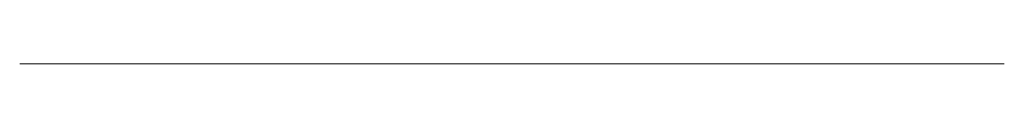
# Model space of a CAD drawing. Units: millimetres. Extents: x 530.6 to 611.6, y 547.2 to 547.2.
import ezdxf

# ---------------------------------------------------------------- set-up
doc = ezdxf.new("R2010")
doc.units = ezdxf.units.MM
doc.layers.add('M-CONS', color=8, linetype='Continuous', lineweight=13)

msp = doc.modelspace()

# ---------------------------------------------------------------- linework, layer by layer
at = {"layer": 'M-CONS'}
for p, q in [((566.633, 547.24, 6), (530.633, 547.24, 6)), ((611.633, 547.24, 6), (566.633, 547.24, 6))]:
    msp.add_line(p, q, dxfattribs=at)

doc.saveas('drawing.dxf')
